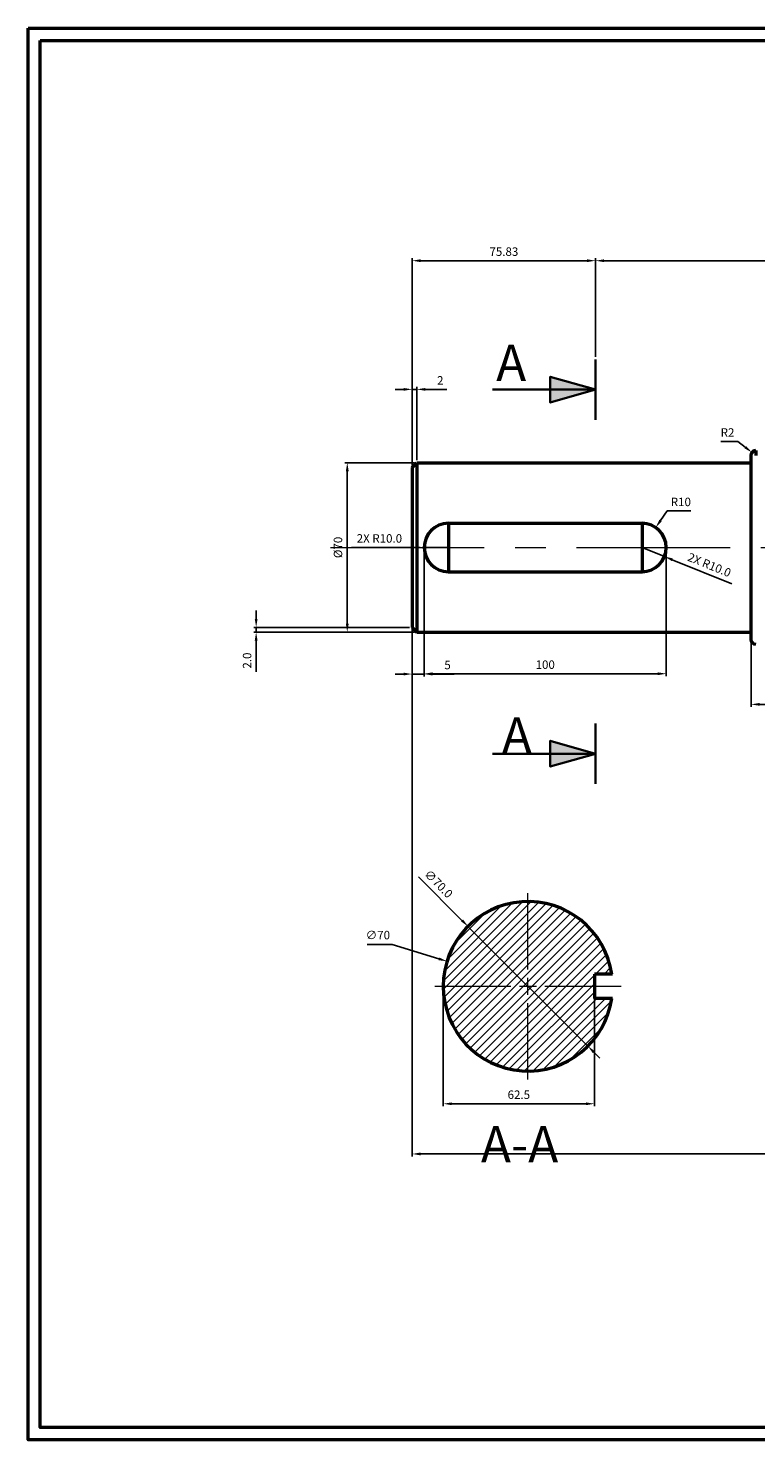
# Model space of a CAD drawing. Units: millimetres. Extents: x 4169 to 4949, y 2556 to 3139.
# Tile 1 of 2: x 4169 to 4470, y 2556 to 3139. Entities that reach past the tile are written whole.
import ezdxf

# ---------------------------------------------------------------- set-up
doc = ezdxf.new("R2010")
doc.units = ezdxf.units.MM
doc.linetypes.add('CENTER', pattern=[50.8, 31.75, -6.35, 6.35, -6.35])
for name, color, linetype, lineweight in [('M-CNTR', 1, 'CENTER', 18), ('M-DIMS', 3, 'Continuous', 25), ('M-HATC', 8, 'Continuous', 18), ('M-OUTL', 7, 'Continuous', 50), ('M-SECT', 7, 'Continuous', 35), ('M-TEXT', 7, 'Continuous', 25), ('M-TTLB', 7, 'Continuous', 50)]:
    doc.layers.add(name, color=color, linetype=linetype, lineweight=lineweight)
doc.styles.get("Standard").update_dxf_attribs({"font": 'arial.ttf'})
doc.dimstyles.new('AM_ISO$0', dxfattribs={"dimtxt": 3.5, "dimasz": 3.5, "dimexe": 1, "dimexo": 1, "dimgap": 1.5, "dimtad": 1, "dimdsep": 46, "dimtxsty": 'Standard', "dimcen": 0, "dimclrd": 256, "dimclre": 256, "dimclrt": 2, "dimadec": 0, "dimazin": 2, "dimtp": 0.1, "dimtm": 0.1, "dimtfac": 0.71, "dimtdec": 3, "dimtmove": 0, "dimatfit": 3, "dimfxl": 1, "dimlwd": -1, "dimlwe": -1, "dimarcsym": 1})
doc.dimstyles.new('AM_ISO$3', dxfattribs={"dimtxt": 3.5, "dimasz": 3.5, "dimexe": 1, "dimexo": 1, "dimgap": 1.5, "dimtad": 1, "dimtoh": 1, "dimdsep": 46, "dimtxsty": 'Standard', "dimcen": 0, "dimclrd": 256, "dimclre": 256, "dimclrt": 2, "dimadec": 0, "dimazin": 2, "dimtp": 0.1, "dimtm": 0.1, "dimtfac": 0.71, "dimtdec": 3, "dimtofl": 0, "dimtmove": 0, "dimatfit": 0, "dimfxl": 1, "dimlwd": -1, "dimlwe": -1, "dimarcsym": 1})
doc.dimstyles.new('AM_ISO$4', dxfattribs={"dimtxt": 3.5, "dimasz": 3.5, "dimexe": 1, "dimexo": 1, "dimgap": 1.5, "dimtad": 1, "dimtoh": 1, "dimdsep": 46, "dimtxsty": 'Standard', "dimcen": 0, "dimclrd": 256, "dimclre": 256, "dimclrt": 2, "dimadec": 0, "dimazin": 2, "dimtp": 0.1, "dimtm": 0.1, "dimtfac": 0.71, "dimtdec": 3, "dimtofl": 0, "dimtmove": 0, "dimatfit": 0, "dimfxl": 1, "dimlwd": -1, "dimlwe": -1, "dimarcsym": 1})

# ---------------------------------------------------------------- blocks, each defined once
blk = doc.blocks.new('*D4')
at = {"layer": 'Defpoints', "color": 0, "transparency": 16777216}
for p in [(4428.31, 2933.25), (4422.64, 2925.01)]:
    blk.add_point(p, dxfattribs=at)
at = {"layer": 'M-DIMS', "color": 0, "linetype": 'ByBlock', "transparency": 16777216}
for p, q in [((4430.29, 2936.13), (4433.01, 2940.08)), ((4433.01, 2940.08), (4442.86, 2940.08))]:
    blk.add_line(p, q, dxfattribs=at)
at = {"layer": 'M-DIMS', "color": 0, "transparency": 16777216}
blk.add_solid([(4429.81, 2936.46), (4430.77, 2935.8), (4428.31, 2933.25)], dxfattribs=at)
at = {"layer": 'M-DIMS', "color": 0, "transparency": 16777216, "insert": (4438.68, 2943.36), "char_height": 3.5, "attachment_point": 5}
blk.add_mtext('R10', dxfattribs=at)
blk = doc.blocks.new('*D7')
at = {"layer": 'Defpoints', "color": 0, "transparency": 16777216}
for p in [(4468.07, 2964.24), (4469.64, 2963.01)]:
    blk.add_point(p, dxfattribs=at)
at = {"layer": 'M-DIMS', "color": 0, "linetype": 'ByBlock', "transparency": 16777216}
for p, q in [((4462.27, 2968.77), (4455.16, 2968.77)), ((4465.31, 2966.39), (4462.27, 2968.77))]:
    blk.add_line(p, q, dxfattribs=at)
at = {"layer": 'M-DIMS', "color": 0, "transparency": 16777216}
blk.add_solid([(4465.67, 2966.85), (4464.95, 2965.94), (4468.07, 2964.24)], dxfattribs=at)
at = {"layer": 'M-DIMS', "color": 0, "transparency": 16777216, "insert": (4457.97, 2972.03), "char_height": 3.5, "attachment_point": 5}
blk.add_mtext('R2', dxfattribs=at)
blk = doc.blocks.new('*D8')
at = {"layer": 'Defpoints', "color": 0, "transparency": 16777216}
for p in [(4329.64, 2990.3), (4327.64, 2958.01), (4329.64, 2960.01)]:
    blk.add_point(p, dxfattribs=at)
at = {"layer": 'M-DIMS', "color": 0, "linetype": 'ByBlock', "transparency": 16777216}
for p, q in [((4327.64, 2959.01), (4327.64, 2991.3)), ((4329.64, 2961.01), (4329.64, 2991.3)), ((4324.14, 2990.3), (4320.64, 2990.3)), ((4327.64, 2990.3), (4329.64, 2990.3)), ((4333.14, 2990.3), (4341.96, 2990.3))]:
    blk.add_line(p, q, dxfattribs=at)
at = {"layer": 'M-DIMS', "color": 0, "transparency": 16777216}
for points in [[(4324.14, 2990.88), (4324.14, 2989.71), (4327.64, 2990.3)], [(4333.14, 2990.88), (4333.14, 2989.71), (4329.64, 2990.3)]]:
    blk.add_solid(points, dxfattribs=at)
at = {"layer": 'M-DIMS', "color": 0, "transparency": 16777216, "insert": (4339.3, 2993.55), "char_height": 3.5, "attachment_point": 5}
blk.add_mtext('2', dxfattribs=at)
blk = doc.blocks.new('*D9')
at = {"layer": 'Defpoints', "color": 0, "transparency": 16777216}
for p in [(4327.64, 2925.01), (4332.64, 2925.01), (4332.64, 2872.72)]:
    blk.add_point(p, dxfattribs=at)
at = {"layer": 'M-DIMS', "color": 0, "linetype": 'ByBlock', "transparency": 16777216}
for p, q in [((4327.64, 2924.01), (4327.64, 2871.72)), ((4332.64, 2924.01), (4332.64, 2871.72)), ((4324.14, 2872.72), (4320.64, 2872.72)), ((4327.64, 2872.72), (4332.64, 2872.72)), ((4336.14, 2872.72), (4344.96, 2872.72))]:
    blk.add_line(p, q, dxfattribs=at)
at = {"layer": 'M-DIMS', "color": 0, "transparency": 16777216}
for points in [[(4324.14, 2873.31), (4324.14, 2872.14), (4327.64, 2872.72)], [(4336.14, 2873.31), (4336.14, 2872.14), (4332.64, 2872.72)]]:
    blk.add_solid(points, dxfattribs=at)
at = {"layer": 'M-DIMS', "color": 0, "transparency": 16777216, "insert": (4342.3, 2876), "char_height": 3.5, "attachment_point": 5}
blk.add_mtext('5', dxfattribs=at)
blk = doc.blocks.new('*D10')
at = {"layer": 'Defpoints', "color": 0, "transparency": 16777216}
for p in [(4332.65, 2925.24), (4432.64, 2925.01), (4432.64, 2872.86)]:
    blk.add_point(p, dxfattribs=at)
at = {"layer": 'M-DIMS', "color": 0, "linetype": 'ByBlock', "transparency": 16777216}
for p, q in [((4332.65, 2924.24), (4332.65, 2871.86)), ((4432.64, 2924.01), (4432.64, 2871.86)), ((4336.15, 2872.86), (4429.14, 2872.86))]:
    blk.add_line(p, q, dxfattribs=at)
at = {"layer": 'M-DIMS', "color": 0, "transparency": 16777216}
for points in [[(4336.15, 2873.44), (4336.15, 2872.27), (4332.65, 2872.86)], [(4429.14, 2873.44), (4429.14, 2872.27), (4432.64, 2872.86)]]:
    blk.add_solid(points, dxfattribs=at)
at = {"layer": 'M-DIMS', "color": 0, "transparency": 16777216, "insert": (4382.65, 2876.15), "char_height": 3.5, "attachment_point": 5}
blk.add_mtext('100', dxfattribs=at)
blk = doc.blocks.new('*D11')
at = {"layer": 'Defpoints', "color": 0, "transparency": 16777216}
for p in [(4467.7, 2886.53), (4551.64, 2882.01), (4551.64, 2860.2)]:
    blk.add_point(p, dxfattribs=at)
at = {"layer": 'M-DIMS', "color": 0, "linetype": 'ByBlock', "transparency": 16777216}
for p, q in [((4467.7, 2885.53), (4467.7, 2859.2)), ((4551.64, 2881.01), (4551.64, 2859.2)), ((4471.2, 2860.2), (4548.14, 2860.2))]:
    blk.add_line(p, q, dxfattribs=at)
at = {"layer": 'M-DIMS', "color": 0, "transparency": 16777216}
for points in [[(4471.2, 2860.79), (4471.2, 2859.62), (4467.7, 2860.2)], [(4548.14, 2860.79), (4548.14, 2859.62), (4551.64, 2860.2)]]:
    blk.add_solid(points, dxfattribs=at)
at = {"layer": 'M-DIMS', "color": 0, "transparency": 16777216, "insert": (4509.67, 2863.49), "char_height": 3.5, "attachment_point": 5}
blk.add_mtext('83.94', dxfattribs=at)
blk = doc.blocks.new('*D14')
at = {"layer": 'Defpoints', "color": 0, "transparency": 16777216}
for p in [(4329.64, 2960.01), (4300.86, 2890.01), (4329.64, 2890.01)]:
    blk.add_point(p, dxfattribs=at)
at = {"layer": 'M-DIMS', "color": 0, "linetype": 'ByBlock', "transparency": 16777216}
for p, q in [((4328.64, 2960.01), (4299.86, 2960.01)), ((4300.86, 2956.51), (4300.86, 2893.51)), ((4328.64, 2890.01), (4299.86, 2890.01))]:
    blk.add_line(p, q, dxfattribs=at)
at = {"layer": 'M-DIMS', "color": 0, "transparency": 16777216}
for points in [[(4300.28, 2956.51), (4301.45, 2956.51), (4300.86, 2960.01)], [(4300.28, 2893.51), (4301.45, 2893.51), (4300.86, 2890.01)]]:
    blk.add_solid(points, dxfattribs=at)
at = {"layer": 'M-DIMS', "color": 0, "transparency": 16777216, "insert": (4297.48, 2925.01), "char_height": 3.5, "attachment_point": 5, "rotation": 90}
blk.add_mtext('%%C70', dxfattribs=at)
blk = doc.blocks.new('*U19')
at = {"layer": 'M-CNTR', "color": 0, "transparency": 16777216}
for p, q in [((0, 7), (0, 38.5)), ((-38.5, 0), (-7, 0)), ((7, 0), (38.5, 0)), ((0, -38.5), (0, -7))]:
    blk.add_line(p, q, dxfattribs=at)
at = {"layer": 'M-CNTR', "color": 0, "linetype": 'Continuous', "transparency": 16777216}
for p, q in [((-3.5, 0), (3.5, 0)), ((0, -3.5), (0, 3.5))]:
    blk.add_line(p, q, dxfattribs=at)
blk = doc.blocks.new('*D20')
at = {"layer": 'Defpoints', "color": 0, "transparency": 16777216}
for p in [(4340.5, 2743.77), (4403, 2743.77), (4340.5, 2695.25)]:
    blk.add_point(p, dxfattribs=at)
at = {"layer": 'M-DIMS', "color": 0, "linetype": 'ByBlock', "transparency": 16777216}
for p, q in [((4340.5, 2742.77), (4340.5, 2694.25)), ((4403, 2742.77), (4403, 2694.25)), ((4399.5, 2695.25), (4344, 2695.25))]:
    blk.add_line(p, q, dxfattribs=at)
at = {"layer": 'M-DIMS', "color": 0, "transparency": 16777216}
for points in [[(4344, 2695.83), (4344, 2694.67), (4340.5, 2695.25)], [(4399.5, 2695.83), (4399.5, 2694.67), (4403, 2695.25)]]:
    blk.add_solid(points, dxfattribs=at)
at = {"layer": 'M-DIMS', "color": 0, "transparency": 16777216, "insert": (4371.75, 2698.54), "char_height": 3.5, "attachment_point": 5}
blk.add_mtext('62.5', dxfattribs=at)
blk = doc.blocks.new('*D21')
at = {"layer": 'Defpoints', "color": 0, "transparency": 16777216}
for p in [(4342.06, 2754.1), (4408.94, 2733.45)]:
    blk.add_point(p, dxfattribs=at)
at = {"layer": 'M-DIMS', "color": 0, "linetype": 'ByBlock', "transparency": 16777216}
for p, q in [((4319.42, 2761.09), (4309.11, 2761.09)), ((4338.71, 2755.13), (4319.42, 2761.09))]:
    blk.add_line(p, q, dxfattribs=at)
at = {"layer": 'M-DIMS', "color": 0, "transparency": 16777216}
blk.add_solid([(4338.89, 2755.69), (4338.54, 2754.57), (4342.06, 2754.1)], dxfattribs=at)
at = {"layer": 'M-DIMS', "color": 0, "transparency": 16777216, "insert": (4313.51, 2764.47), "char_height": 3.5, "attachment_point": 5}
blk.add_mtext('∅70', dxfattribs=at)
blk = doc.blocks.new('*D24')
at = {"layer": 'Defpoints', "color": 0, "transparency": 16777216}
for p in [(4327.64, 2892.01), (4797.64, 2887.01), (4797.64, 2674.52)]:
    blk.add_point(p, dxfattribs=at)
at = {"layer": 'M-DIMS', "linetype": 'ByBlock', "transparency": 16777216}
for p, q in [((4327.64, 2891.01), (4327.64, 2673.52)), ((4797.64, 2886.01), (4797.64, 2673.52)), ((4331.14, 2674.52), (4794.14, 2674.52))]:
    blk.add_line(p, q, dxfattribs=at)
at = {"layer": 'M-DIMS', "transparency": 16777216}
for points in [[(4331.14, 2675.11), (4331.14, 2673.94), (4327.64, 2674.52)], [(4794.14, 2675.11), (4794.14, 2673.94), (4797.64, 2674.52)]]:
    blk.add_solid(points, dxfattribs=at)
at = {"layer": 'M-DIMS', "color": 2, "transparency": 16777216, "insert": (4562.64, 2677.81), "char_height": 3.5, "attachment_point": 5}
blk.add_mtext('470.0', dxfattribs=at)
blk = doc.blocks.new('*D26')
at = {"layer": 'Defpoints', "color": 0, "transparency": 16777216}
for p in [(4403.47, 3043.44), (4403.47, 3002.69), (4327.64, 2958.01)]:
    blk.add_point(p, dxfattribs=at)
at = {"layer": 'M-DIMS', "linetype": 'ByBlock', "transparency": 16777216}
for p, q in [((4327.64, 2959.01), (4327.64, 3044.44)), ((4331.14, 3043.44), (4399.97, 3043.44)), ((4403.47, 3003.69), (4403.47, 3044.44))]:
    blk.add_line(p, q, dxfattribs=at)
at = {"layer": 'M-DIMS', "transparency": 16777216}
for points in [[(4331.14, 3044.02), (4331.14, 3042.86), (4327.64, 3043.44)], [(4399.97, 3044.02), (4399.97, 3042.86), (4403.47, 3043.44)]]:
    blk.add_solid(points, dxfattribs=at)
at = {"layer": 'M-DIMS', "color": 2, "transparency": 16777216, "insert": (4365.56, 3046.73), "char_height": 3.5, "attachment_point": 5}
blk.add_mtext('75.83', dxfattribs=at)
blk = doc.blocks.new('*D27')
at = {"layer": 'Defpoints', "color": 0, "transparency": 16777216}
for p in [(4634.66, 3043.44), (4403.47, 3002.69), (4634.66, 3000.19)]:
    blk.add_point(p, dxfattribs=at)
at = {"layer": 'M-DIMS', "linetype": 'ByBlock', "transparency": 16777216}
for p, q in [((4403.47, 3003.69), (4403.47, 3044.44)), ((4406.97, 3043.44), (4631.16, 3043.44)), ((4634.66, 3001.19), (4634.66, 3044.44))]:
    blk.add_line(p, q, dxfattribs=at)
at = {"layer": 'M-DIMS', "transparency": 16777216}
for points in [[(4406.97, 3044.02), (4406.97, 3042.86), (4403.47, 3043.44)], [(4631.16, 3044.02), (4631.16, 3042.86), (4634.66, 3043.44)]]:
    blk.add_solid(points, dxfattribs=at)
at = {"layer": 'M-DIMS', "color": 2, "transparency": 16777216, "insert": (4519.06, 3046.73), "char_height": 3.5, "attachment_point": 5}
blk.add_mtext('231.2', dxfattribs=at)
blk = doc.blocks.new('*D28')
at = {"layer": 'Defpoints', "color": 0, "transparency": 16777216}
for p in [(4422.64, 2925.01), (4431.92, 2921.26)]:
    blk.add_point(p, dxfattribs=at)
at = {"layer": 'M-DIMS', "linetype": 'ByBlock', "transparency": 16777216}
for p, q in [((4422.64, 2925.01), (4431.92, 2921.26)), ((4459.74, 2910.03), (4435.16, 2919.95))]:
    blk.add_line(p, q, dxfattribs=at)
at = {"layer": 'M-DIMS', "transparency": 16777216}
blk.add_solid([(4435.38, 2920.49), (4434.94, 2919.41), (4431.92, 2921.26)], dxfattribs=at)
at = {"layer": 'M-DIMS', "color": 2, "transparency": 16777216, "insert": (4450.31, 2917.38), "char_height": 3.5, "attachment_point": 5, "rotation": 338.01633}
blk.add_mtext('2X R10.0', dxfattribs=at)
blk = doc.blocks.new('*D32')
at = {"layer": 'Defpoints', "color": 0, "transparency": 16777216}
for p in [(4350.74, 2768.51), (4400.26, 2719.04)]:
    blk.add_point(p, dxfattribs=at)
at = {"layer": 'M-DIMS', "linetype": 'ByBlock', "transparency": 16777216}
for p, q in [((4330.26, 2788.97), (4348.26, 2770.98)), ((4400.26, 2719.04), (4350.74, 2768.51)), ((4402.74, 2716.56), (4405.21, 2714.09))]:
    blk.add_line(p, q, dxfattribs=at)
at = {"layer": 'M-DIMS', "transparency": 16777216}
for points in [[(4348.68, 2771.4), (4347.85, 2770.57), (4350.74, 2768.51)], [(4403.15, 2716.98), (4402.33, 2716.15), (4400.26, 2719.04)]]:
    blk.add_solid(points, dxfattribs=at)
at = {"layer": 'M-DIMS', "color": 2, "transparency": 16777216, "insert": (4338.28, 2785.75), "char_height": 3.5, "attachment_point": 5, "rotation": 315.02784}
blk.add_mtext('∅70.0', dxfattribs=at)
blk = doc.blocks.new('*D33')
at = {"layer": 'Defpoints', "color": 0, "transparency": 16777216}
for p in [(4327.64, 2892.01), (4263.22, 2890.01), (4329.64, 2890.01)]:
    blk.add_point(p, dxfattribs=at)
at = {"layer": 'M-DIMS', "linetype": 'ByBlock', "transparency": 16777216}
for p, q in [((4263.22, 2895.51), (4263.22, 2899.01)), ((4326.64, 2892.01), (4262.22, 2892.01)), ((4263.22, 2892.01), (4263.22, 2890.01)), ((4328.64, 2890.01), (4262.22, 2890.01)), ((4263.22, 2886.51), (4263.22, 2873.59))]:
    blk.add_line(p, q, dxfattribs=at)
at = {"layer": 'M-DIMS', "transparency": 16777216}
for points in [[(4262.63, 2895.51), (4263.8, 2895.51), (4263.22, 2892.01)], [(4262.63, 2886.51), (4263.8, 2886.51), (4263.22, 2890.01)]]:
    blk.add_solid(points, dxfattribs=at)
at = {"layer": 'M-DIMS', "color": 2, "transparency": 16777216, "insert": (4259.93, 2878.3), "char_height": 3.5, "attachment_point": 5, "rotation": 90}
blk.add_mtext('2.0', dxfattribs=at)
blk = doc.blocks.new('*D34')
at = {"layer": 'Defpoints', "color": 0, "transparency": 16777216}
for p in [(4332.64, 2925.01), (4342.64, 2925.01)]:
    blk.add_point(p, dxfattribs=at)
at = {"layer": 'M-DIMS', "linetype": 'ByBlock', "transparency": 16777216}
for p, q in [((4302.63, 2925.01), (4329.14, 2925.01)), ((4342.64, 2925.01), (4332.64, 2925.01))]:
    blk.add_line(p, q, dxfattribs=at)
at = {"layer": 'M-DIMS', "transparency": 16777216}
blk.add_solid([(4329.14, 2925.59), (4329.14, 2924.42), (4332.64, 2925.01)], dxfattribs=at)
at = {"layer": 'M-DIMS', "color": 2, "transparency": 16777216, "insert": (4314.14, 2928.29), "char_height": 3.5, "attachment_point": 5, "rotation": 359.99751}
blk.add_mtext('2X R10.0', dxfattribs=at)

msp = doc.modelspace()

# ---------------------------------------------------------------- hatches: boundary and pattern name
at = {"layer": 'M-HATC'}
h = msp.add_hatch(dxfattribs=at)
h.set_pattern_fill('_U', color=256, scale=2.5, angle=45, style=0, pattern_type=0)
h.set_pattern_definition([(45, (0, 0), (-1.767767, 1.767767), [])])
edge = h.paths.add_edge_path()
edge.add_line((4410.142, 2738.773), (4403.001, 2738.773))
edge.add_line((4403.001, 2738.773), (4403.001, 2748.773))
edge.add_line((4403.001, 2748.773), (4410.142, 2748.773))
edge.add_arc((4375.501, 2743.773), 35, 8.213211, 351.786789)
at = {"layer": 'M-SECT'}
h = msp.add_hatch(color=256, dxfattribs=at)
h.set_gradient(color1=(0, 0, 255), color2=(255, 255, 0), tint=1, name='CYLINDER')
h.paths.add_polyline_path([(4403.47, 2990.189), (4384.746, 2990.189), (4384.746, 2984.843)])
h.paths.add_polyline_path([(4384.746, 2995.535), (4384.746, 2990.189), (4403.47, 2990.189)])
h.paths.add_polyline_path([(4384.746, 2845.17), (4384.746, 2839.824), (4403.47, 2839.824)])
h.paths.add_polyline_path([(4403.47, 2839.824), (4384.746, 2839.824), (4384.746, 2834.478)])

# ---------------------------------------------------------------- linework, layer by layer
at = {"layer": 'M-CNTR', "ltscale": 2}
msp.add_line((4293.966, 2925.007), (4850.492, 2925.007), dxfattribs=at)
at = {"layer": 'M-OUTL'}
for p, q in [((4467.644, 2963.007), (4467.644, 2887.007)), ((4469.644, 2965.007), (4469.644, 2963.007)), ((4327.644, 2958.007), (4329.644, 2960.007)), ((4327.644, 2958.007), (4327.644, 2892.007)), ((4329.644, 2960.007), (4467.644, 2960.007)), ((4329.644, 2960.007), (4329.644, 2890.007)), ((4342.644, 2935.007), (4342.644, 2915.007)), ((4342.644, 2935.007), (4422.644, 2935.007)), ((4422.644, 2935.007), (4422.644, 2915.007)), ((4342.644, 2915.007), (4422.644, 2915.007)), ((4327.644, 2892.007), (4329.644, 2890.007)), ((4329.644, 2890.007), (4467.644, 2890.007)), ((4410.501, 2748.773), (4403.001, 2748.773)), ((4403.001, 2748.773), (4403.001, 2738.773)), ((4410.501, 2738.773), (4403.001, 2738.773)), ((4410.501, 2738.773), (4403.001, 2738.773))]:
    msp.add_line(p, q, dxfattribs=at)
for centre, radius, start, end in [((4469.644, 2963.007), 2, 90, 180), ((4342.644, 2925.007), 10, 90, 270), ((4422.644, 2925.007), 10, 270, 90), ((4469.644, 2887.007), 2, 180, 270), ((4375.501, 2743.773), 35, 8.213211, 351.786789)]:
    msp.add_arc(centre, radius, start, end, dxfattribs=at)
at = {"layer": 'M-SECT'}
for p, q in [((4403.47, 3002.689), (4403.47, 2977.689)), ((4403.47, 2990.189), (4360.884, 2990.189)), ((4403.47, 2990.189), (4372.095, 2990.189)), ((4403.47, 2827.324), (4403.47, 2852.324)), ((4403.47, 2839.824), (4360.884, 2839.824))]:
    msp.add_line(p, q, dxfattribs=at)
for points in [[(4403.47, 2990.189), (4384.746, 2995.535), (4384.746, 2984.843)], [(4403.47, 2839.824), (4384.746, 2845.17), (4384.746, 2834.478)]]:
    msp.add_lwpolyline(points, close=True, dxfattribs=at)
at = {"layer": 'M-TTLB'}
for points in [[(4169.043, 3139.451), (4948.587, 3139.451), (4948.587, 2556.482), (4169.043, 2556.482)], [(4174.043, 3134.451), (4943.587, 3134.451), (4943.587, 2561.482), (4174.043, 2561.482)]]:
    msp.add_lwpolyline(points, close=True, dxfattribs=at)

# ---------------------------------------------------------------- block references
at = {"layer": 'M-CNTR'}
msp.add_blockref('*U19', (4375.501, 2743.773), dxfattribs=at)

# ---------------------------------------------------------------- texts
at = {"layer": 'M-TEXT'}
for s, p in [('A', (4362.368, 2993.704)), ('A', (4364.707, 2839.824)), ('A-A', (4356.063, 2671.015))]:
    msp.add_text(s, height=15, dxfattribs=at).set_placement(p)

# ---------------------------------------------------------------- dimensions: what is measured, and where the dimension line sits
at = {"layer": 'M-DIMS'}
for base, p1, p2, override, picture, middle in [((4403.47, 3043.439), (4327.644, 2958.007), (4403.47, 3002.689), {"dimdec": 2, "dimlfac": 1, "dimrnd": 0, "dimzin": 0, "dimdsep": 46, "dimlunit": 2}, '*D26', (4365.557, 3046.727)), ((4634.658, 3043.439), (4403.47, 3002.689), (4634.658, 3000.189), {"dimdec": 1, "dimlfac": 1, "dimrnd": 0, "dimzin": 0, "dimdsep": 46, "dimlunit": 2}, '*D27', (4519.064, 3046.727)), ((4329.644, 2990.295), (4327.644, 2958.007), (4329.644, 2960.007), {"dimpost": '', "dimclrd": 0, "dimclre": 0, "dimclrt": 0}, '*D8', (4339.303, 2993.552)), ((4797.644, 2674.523), (4327.644, 2892.007), (4797.644, 2887.007), {"dimdec": 1, "dimlfac": 1, "dimrnd": 0, "dimzin": 0, "dimdsep": 46, "dimlunit": 2}, '*D24', (4562.644, 2677.81))]:
    dim = msp.add_linear_dim(base=base, p1=p1, p2=p2, dimstyle='AM_ISO$0', override=override, dxfattribs=at)
    dim.commit()
    dim.dimension.update_dxf_attribs({"geometry": picture, "text_midpoint": middle})
for center, mpoint, override, picture, middle in [((4469.644, 2963.007), (4468.068, 2964.239), {"dimclrd": 0, "dimclre": 0, "dimclrt": 0}, '*D7', (4457.968, 2968.771)), ((4422.644, 2925.007), (4428.31, 2933.247), {"dimpost": '', "dimclrd": 0, "dimclre": 0, "dimclrt": 0}, '*D4', (4438.681, 2940.076))]:
    dim = msp.add_radius_dim(center=center, mpoint=mpoint, dimstyle='AM_ISO$4', override=override, dxfattribs=at)
    dim.commit()
    dim.dimension.update_dxf_attribs({"geometry": picture, "text_midpoint": middle, "dimtype": 164})
dim = msp.add_linear_dim(base=(4300.864, 2890.007), p1=(4329.644, 2960.007), p2=(4329.644, 2890.007), angle=90, text='%%C<>', dimstyle='AM_ISO$0', override={"dimpost": '', "dimclrd": 0, "dimclre": 0, "dimclrt": 0}, dxfattribs=at)
dim.commit()
dim.dimension.update_dxf_attribs({"geometry": '*D14', "text_midpoint": (4297.479, 2925.007)})
for center, mpoint, picture, middle in [((4342.644, 2925.007), (4332.644, 2925.007), '*D34', (4314.139, 2928.295)), ((4422.644, 2925.007), (4431.917, 2921.263), '*D28', (4450.306, 2917.384))]:
    dim = msp.add_radius_dim(center=center, mpoint=mpoint, text='2X <>', dimstyle='AM_ISO$0', override={"dimdec": 1, "dimlfac": 1, "dimrnd": 0, "dimzin": 0, "dimdsep": 46, "dimlunit": 2}, dxfattribs=at)
    dim.commit()
    dim.dimension.update_dxf_attribs({"geometry": picture, "text_midpoint": middle})
for base, p1, p2, angle, override, picture, middle in [((4332.644, 2872.724), (4327.644, 2925.007), (4332.644, 2925.007), 0, {"dimpost": '', "dimclrd": 0, "dimclre": 0, "dimclrt": 0}, '*D9', (4342.304, 2876.004)), ((4432.644, 2872.858), (4332.647, 2925.242), (4432.644, 2925.007), 0, {"dimclrd": 0, "dimclre": 0, "dimclrt": 0}, '*D10', (4382.645, 2876.145)), ((4263.216, 2890.007), (4327.644, 2892.007), (4329.644, 2890.007), 90, {"dimdec": 1, "dimlfac": 1, "dimrnd": 0, "dimzin": 0, "dimdsep": 46, "dimlunit": 2}, '*D33', (4259.928, 2878.297)), ((4551.644, 2860.204), (4467.701, 2886.531), (4551.644, 2882.007), 0, {"dimpost": '', "dimclrd": 0, "dimclre": 0, "dimclrt": 0}, '*D11', (4509.673, 2863.492))]:
    dim = msp.add_linear_dim(base=base, p1=p1, p2=p2, angle=angle, dimstyle='AM_ISO$0', override=override, dxfattribs=at)
    dim.commit()
    dim.dimension.update_dxf_attribs({"geometry": picture, "text_midpoint": middle})
for p1, p2, dimstyle, override, picture, middle in [((4400.262, 2719.036), (4350.74, 2768.51), 'AM_ISO$0', {"dimdec": 1, "dimlfac": 1, "dimrnd": 0, "dimzin": 0, "dimdsep": 46, "dimlunit": 2}, '*D32', (4335.884, 2783.352)), ((4408.944, 2733.447), (4342.059, 2754.098), 'AM_ISO$3', {"dimpost": '', "dimclrd": 0, "dimclre": 0, "dimclrt": 0}, '*D21', (4313.513, 2761.089))]:
    dim = msp.add_diameter_dim_2p(p1=p1, p2=p2, dimstyle=dimstyle, override=override, dxfattribs=at)
    dim.commit()
    dim.dimension.update_dxf_attribs({"geometry": picture, "text_midpoint": middle, "dimtype": 163})
dim = msp.add_linear_dim(base=(4340.501, 2695.251), p1=(4403.001, 2743.773), p2=(4340.501, 2743.773), dimstyle='AM_ISO$0', override={"dimclrd": 0, "dimclre": 0, "dimclrt": 0}, dxfattribs=at)
dim.commit()
dim.dimension.update_dxf_attribs({"geometry": '*D20', "text_midpoint": (4371.751, 2695.251), "dimtype": 160})

doc.saveas('drawing.dxf')
